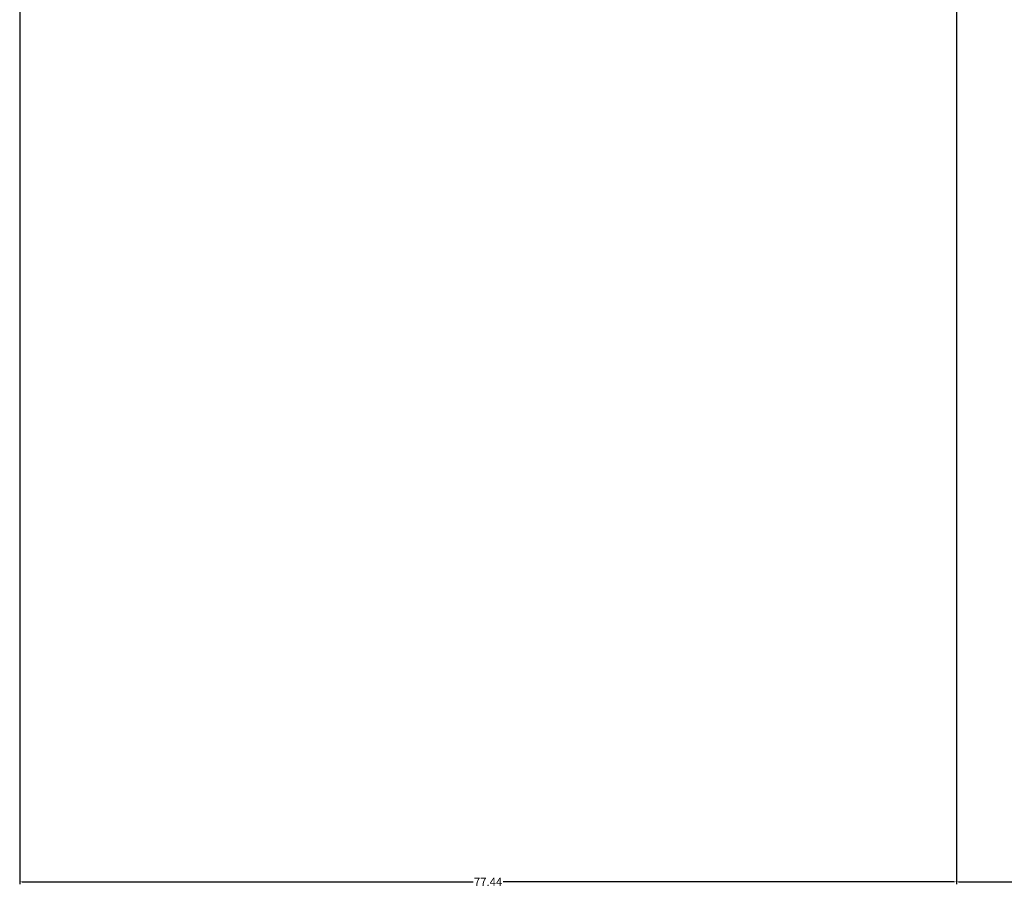
# Model space of a CAD drawing. Units: inches. Extents: x -145 to 510, y 5 to 386.
# Tile 1 of 25: x -62 to 20, y 5 to 77. Entities that reach past the tile are written whole.
import ezdxf

# ---------------------------------------------------------------- set-up
doc = ezdxf.new("R2010")
doc.units = ezdxf.units.IN
doc.header["$MEASUREMENT"] = 0
doc.layers.add('A-ANNO-DIMS', color=2, linetype='Continuous', lineweight=18)
doc.styles.get("Standard").update_dxf_attribs({"font": 'arial.ttf'})
doc.dimstyles.get("Standard").update_dxf_attribs({"dimtxt": 0.6875, "dimasz": 0.18, "dimexe": 0.18, "dimexo": 0.0625, "dimgap": 0.09, "dimtad": 0, "dimtih": 1, "dimtoh": 1, "dimdec": 4, "dimzin": 0, "dimdsep": 46, "dimlunit": 4, "dimtxsty": 'Standard', "dimcen": 0.09, "dimadec": 0, "dimazin": 0, "dimtfac": 1, "dimtdec": 4, "dimtofl": 0, "dimtmove": 0, "dimatfit": 3, "dimfxl": 1, "dimtolj": 1, "dimtzin": 0, "dimarcsym": 0})

# ---------------------------------------------------------------- blocks, each defined once
blk = doc.blocks.new('*D40')
at = {"layer": 'A-ANNO-DIMS', "color": 0, "lineweight": -2, "transparency": 16777216}
for p, q in [((-61.692, 109.056), (-61.692, 5.194)), ((15.744, 109.056), (15.744, 5.194)), ((-61.512, 5.374), (-24.22, 5.374)), ((15.564, 5.374), (-21.728, 5.374))]:
    blk.add_line(p, q, dxfattribs=at)
at = {"layer": 'A-ANNO-DIMS', "color": 0, "transparency": 16777216}
for points in [[(-61.512, 5.404), (-61.512, 5.344), (-61.692, 5.374)], [(15.564, 5.404), (15.564, 5.344), (15.744, 5.374)]]:
    blk.add_solid(points, dxfattribs=at)
at = {"layer": 'Defpoints', "color": 0, "transparency": 16777216}
for p in [(-61.692, 109.118), (15.744, 109.118), (15.744, 5.374)]:
    blk.add_point(p, dxfattribs=at)
at = {"layer": 'A-ANNO-DIMS', "color": 0, "transparency": 16777216, "insert": (-22.974, 5.374), "char_height": 0.6875, "attachment_point": 5}
blk.add_mtext('\\A1;77.44', dxfattribs=at)
blk = doc.blocks.new('*D41')
at = {"layer": 'A-ANNO-DIMS', "color": 0, "lineweight": -2, "transparency": 16777216}
for p, q in [((15.744, 109.056), (15.744, 5.194)), ((54.001, 79.828), (54.001, 5.194)), ((15.924, 5.374), (33.623, 5.374)), ((53.821, 5.374), (36.122, 5.374))]:
    blk.add_line(p, q, dxfattribs=at)
at = {"layer": 'A-ANNO-DIMS', "color": 0, "transparency": 16777216}
for points in [[(15.924, 5.404), (15.924, 5.344), (15.744, 5.374)], [(53.821, 5.404), (53.821, 5.344), (54.001, 5.374)]]:
    blk.add_solid(points, dxfattribs=at)
at = {"layer": 'Defpoints', "color": 0, "transparency": 16777216}
for p in [(15.744, 109.118), (54.001, 79.891), (54.001, 5.374)]:
    blk.add_point(p, dxfattribs=at)
at = {"layer": 'A-ANNO-DIMS', "color": 0, "transparency": 16777216, "insert": (34.873, 5.374), "char_height": 0.6875, "attachment_point": 5}
blk.add_mtext('\\A1;38.26', dxfattribs=at)

msp = doc.modelspace()

# ---------------------------------------------------------------- dimensions: what is measured, and where the dimension line sits
at = {"layer": 'A-ANNO-DIMS'}
for base, p1, p2, picture, middle in [((15.7444, 5.3738), (-61.6923, 109.1183), (15.7444, 109.1183), '*D40', (-22.9739, 5.3738)), ((54.0014, 5.3738), (15.7444, 109.1183), (54.0014, 79.8905), '*D41', (34.8729, 5.3738))]:
    dim = msp.add_linear_dim(base=base, p1=p1, p2=p2, dimstyle='Standard', override={"dimdec": 2, "dimlfac": 1, "dimrnd": 0, "dimzin": 0, "dimdsep": 46, "dimlunit": 2}, dxfattribs=at)
    dim.commit()
    dim.dimension.update_dxf_attribs({"geometry": picture, "text_midpoint": middle})

doc.saveas('drawing.dxf')
